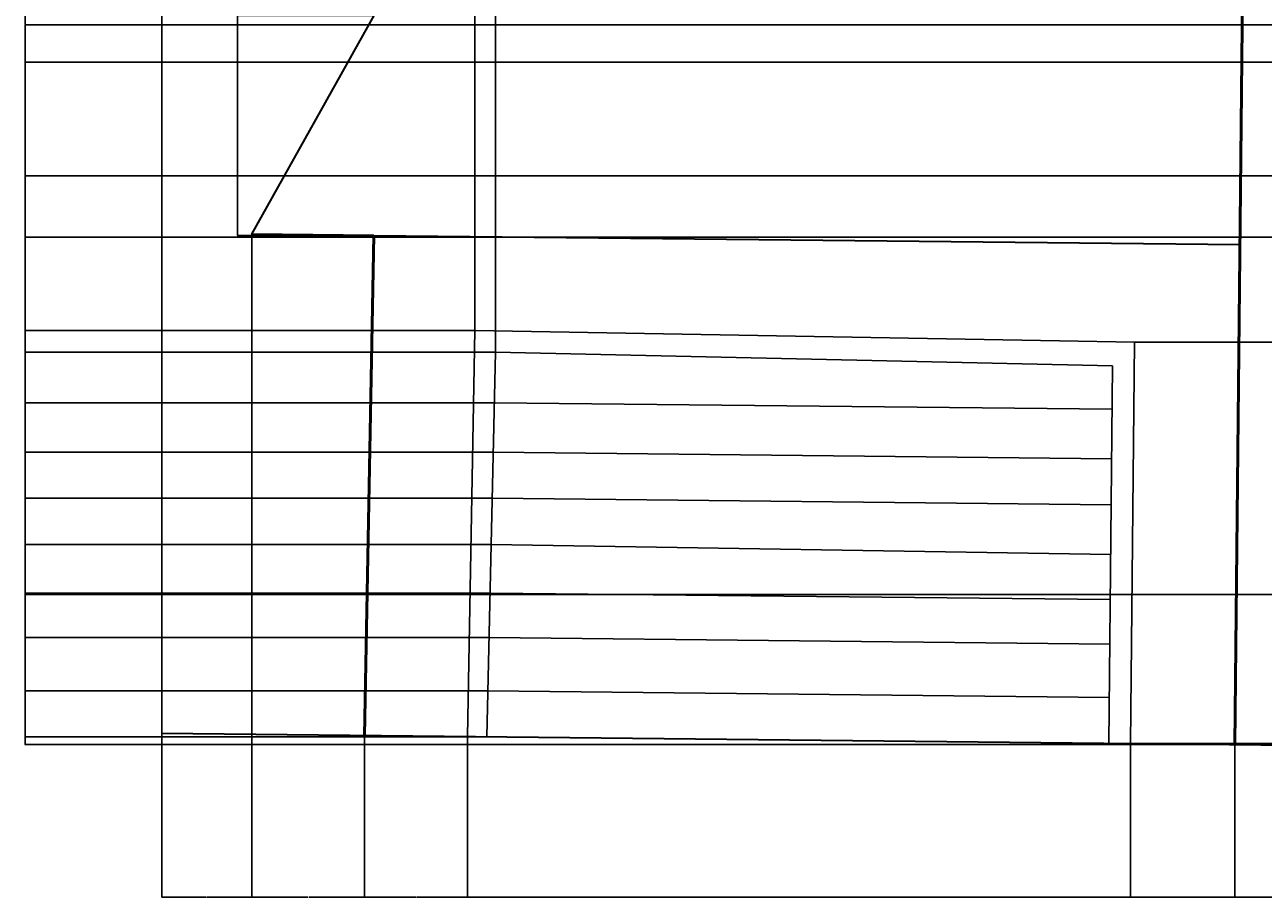
# Model space of a CAD drawing. Units: millimetres. Extents: x 1119 to 4262, y 854 to 2737.
# Tile 1 of 5: x 1119 to 2434, y 854 to 1780. Entities that reach past the tile are written whole.
import ezdxf

# ---------------------------------------------------------------- set-up
doc = ezdxf.new("R2010")
doc.units = ezdxf.units.MM
for name, color, linetype, lineweight in [('A-ANNO-DIMS', 2, 'Continuous', 18), ('A-DOOR', 3, 'Continuous', 25), ('A-ELEV', 8, 'Continuous', 35), ('A-ROOF', 1, 'Continuous', 35), ('A-WALL', 7, 'Continuous', 50)]:
    doc.layers.add(name, color=color, linetype=linetype, lineweight=lineweight)
doc.styles.get("Standard").update_dxf_attribs({"font": 'arial.ttf'})
doc.dimstyles.get("Standard").update_dxf_attribs({"dimtxt": 0.18, "dimasz": 0.18, "dimexe": 0.18, "dimexo": 0.0625, "dimgap": 0.09, "dimtad": 0, "dimtih": 1, "dimtoh": 1, "dimdec": 4, "dimzin": 0, "dimdsep": 46, "dimtxsty": 'Standard', "dimcen": 0.09, "dimadec": 0, "dimazin": 0, "dimtfac": 1, "dimtdec": 4, "dimtofl": 0, "dimtmove": 0, "dimatfit": 3, "dimfxl": 1, "dimtolj": 1, "dimtzin": 0, "dimarcsym": 0})

# ---------------------------------------------------------------- blocks, each defined once
blk = doc.blocks.new('*D1')
at = {"layer": 'A-ANNO-DIMS', "color": 0, "lineweight": -2, "transparency": 16777216}
for p, q in [((1360.1, 1558), (1360.1, 854.2)), ((1264.4, 1028.1), (1264.4, 854.2)), ((1264.5, 854.4), (1311.9, 854.4)), ((1360, 854.4), (1312.6, 854.4))]:
    blk.add_line(p, q, dxfattribs=at)
at = {"layer": 'A-ANNO-DIMS', "color": 0, "transparency": 16777216}
for points in [[(1264.5, 854.4), (1264.5, 854.3), (1264.4, 854.4)], [(1360, 854.4), (1360, 854.3), (1360.1, 854.4)]]:
    blk.add_solid(points, dxfattribs=at)
at = {"layer": 'Defpoints', "color": 0, "transparency": 16777216}
for p in [(1360.1, 1558.1), (1264.4, 1028.2), (1360.1, 854.4)]:
    blk.add_point(p, dxfattribs=at)
at = {"layer": 'A-ANNO-DIMS', "color": 0, "transparency": 16777216, "insert": (1312.2, 854.4), "char_height": 0.18, "attachment_point": 5}
blk.add_mtext('\\A1;95.78', dxfattribs=at)
blk = doc.blocks.new('*D2')
at = {"layer": 'A-ANNO-DIMS', "color": 0, "lineweight": -2, "transparency": 16777216}
for p, q in [((1360.1, 1558), (1360.1, 854.2)), ((1479.9, 1025.9), (1479.9, 854.2)), ((1360.3, 854.4), (1419.6, 854.4)), ((1479.7, 854.4), (1420.5, 854.4))]:
    blk.add_line(p, q, dxfattribs=at)
at = {"layer": 'A-ANNO-DIMS', "color": 0, "transparency": 16777216}
for points in [[(1360.3, 854.4), (1360.3, 854.3), (1360.1, 854.4)], [(1479.7, 854.4), (1479.7, 854.3), (1479.9, 854.4)]]:
    blk.add_solid(points, dxfattribs=at)
at = {"layer": 'Defpoints', "color": 0, "transparency": 16777216}
for p in [(1360.1, 1558.1), (1479.9, 1025.9), (1479.9, 854.4)]:
    blk.add_point(p, dxfattribs=at)
at = {"layer": 'A-ANNO-DIMS', "color": 0, "transparency": 16777216, "insert": (1420, 854.4), "char_height": 0.18, "attachment_point": 5}
blk.add_mtext('\\A1;119.76', dxfattribs=at)
blk = doc.blocks.new('*D3')
at = {"layer": 'A-ANNO-DIMS', "color": 0, "lineweight": -2, "transparency": 16777216}
for p, q in [((1479.9, 1025.9), (1479.9, 854.2)), ((1589.2, 1024.7), (1589.2, 854.2)), ((1480.1, 854.4), (1534.1, 854.4)), ((1589, 854.4), (1535, 854.4))]:
    blk.add_line(p, q, dxfattribs=at)
at = {"layer": 'A-ANNO-DIMS', "color": 0, "transparency": 16777216}
for points in [[(1480.1, 854.4), (1480.1, 854.3), (1479.9, 854.4)], [(1589, 854.4), (1589, 854.3), (1589.2, 854.4)]]:
    blk.add_solid(points, dxfattribs=at)
at = {"layer": 'Defpoints', "color": 0, "transparency": 16777216}
for p in [(1479.9, 1025.9), (1589.2, 1024.8), (1589.2, 854.4)]:
    blk.add_point(p, dxfattribs=at)
at = {"layer": 'A-ANNO-DIMS', "color": 0, "transparency": 16777216, "insert": (1534.6, 854.4), "char_height": 0.18, "attachment_point": 5}
blk.add_mtext('\\A1;109.32', dxfattribs=at)
blk = doc.blocks.new('*D4')
at = {"layer": 'A-ANNO-DIMS', "color": 0, "lineweight": -2, "transparency": 16777216}
for p, q in [((1589.2, 1024.7), (1589.2, 854.2)), ((2403.9, 1016.1), (2403.9, 854.2)), ((1589.4, 854.4), (1996.2, 854.4)), ((2403.7, 854.4), (1997, 854.4))]:
    blk.add_line(p, q, dxfattribs=at)
at = {"layer": 'A-ANNO-DIMS', "color": 0, "transparency": 16777216}
for points in [[(1589.4, 854.4), (1589.4, 854.3), (1589.2, 854.4)], [(2403.7, 854.4), (2403.7, 854.3), (2403.9, 854.4)]]:
    blk.add_solid(points, dxfattribs=at)
at = {"layer": 'Defpoints', "color": 0, "transparency": 16777216}
for p in [(1589.2, 1024.8), (2403.9, 1016.2), (2403.9, 854.4)]:
    blk.add_point(p, dxfattribs=at)
at = {"layer": 'A-ANNO-DIMS', "color": 0, "transparency": 16777216, "insert": (1996.6, 854.4), "char_height": 0.18, "attachment_point": 5}
blk.add_mtext('\\A1;814.7', dxfattribs=at)
blk = doc.blocks.new('*D5')
at = {"layer": 'A-ANNO-DIMS', "color": 0, "lineweight": -2, "transparency": 16777216}
for p, q in [((2537.2, 1175.4), (2537.2, 854.2)), ((2403.9, 1016.1), (2403.9, 854.2)), ((2404.1, 854.4), (2470.2, 854.4)), ((2537, 854.4), (2470.9, 854.4))]:
    blk.add_line(p, q, dxfattribs=at)
at = {"layer": 'A-ANNO-DIMS', "color": 0, "transparency": 16777216}
for points in [[(2404.1, 854.4), (2404.1, 854.3), (2403.9, 854.4)], [(2537, 854.4), (2537, 854.3), (2537.2, 854.4)]]:
    blk.add_solid(points, dxfattribs=at)
at = {"layer": 'Defpoints', "color": 0, "transparency": 16777216}
for p in [(2537.2, 1175.4), (2403.9, 1016.2), (2537.2, 854.4)]:
    blk.add_point(p, dxfattribs=at)
at = {"layer": 'A-ANNO-DIMS', "color": 0, "transparency": 16777216, "insert": (2470.5, 854.4), "char_height": 0.18, "attachment_point": 5}
blk.add_mtext('\\A1;133.3', dxfattribs=at)
blk = doc.blocks.new('*D13')
at = {"layer": 'A-ANNO-DIMS', "color": 0, "lineweight": -2, "transparency": 16777216}
for p, q in [((1264.4, 1028.3), (1264.4, 2737.1)), ((1264.5, 2737), (2690.1, 2737)), ((4116.6, 2737), (2691, 2737)), ((4116.8, 2249.8), (4116.8, 2737.1))]:
    blk.add_line(p, q, dxfattribs=at)
at = {"layer": 'A-ANNO-DIMS', "color": 0, "transparency": 16777216}
for points in [[(1264.5, 2737), (1264.5, 2736.9), (1264.4, 2737)], [(4116.6, 2737), (4116.6, 2736.9), (4116.8, 2737)]]:
    blk.add_solid(points, dxfattribs=at)
at = {"layer": 'Defpoints', "color": 0, "transparency": 16777216}
for p in [(4116.8, 2737), (4116.8, 2249.7), (1264.4, 1028.2)]:
    blk.add_point(p, dxfattribs=at)
at = {"layer": 'A-ANNO-DIMS', "color": 0, "transparency": 16777216, "insert": (2690.6, 2737), "char_height": 0.18, "attachment_point": 5}
blk.add_mtext('\\A1;2852.4', dxfattribs=at)
blk = doc.blocks.new('*D31')
at = {"layer": 'A-ANNO-DIMS', "color": 0, "lineweight": -2, "transparency": 16777216}
for p, q in [((2537.1, 1175.4), (1119.2, 1175.4)), ((1119.4, 1175.3), (1119.4, 1096)), ((1119.4, 1016.4), (1119.4, 1095.6)), ((2403.8, 1016.2), (1119.2, 1016.2))]:
    blk.add_line(p, q, dxfattribs=at)
at = {"layer": 'A-ANNO-DIMS', "color": 0, "transparency": 16777216}
for points in [[(1119.3, 1175.3), (1119.4, 1175.3), (1119.4, 1175.4)], [(1119.3, 1016.4), (1119.4, 1016.4), (1119.4, 1016.2)]]:
    blk.add_solid(points, dxfattribs=at)
at = {"layer": 'Defpoints', "color": 0, "transparency": 16777216}
for p in [(1119.4, 1175.4), (2537.2, 1175.4), (2403.9, 1016.2)]:
    blk.add_point(p, dxfattribs=at)
at = {"layer": 'A-ANNO-DIMS', "color": 0, "transparency": 16777216, "insert": (1119.4, 1095.8), "char_height": 0.18, "attachment_point": 5}
blk.add_mtext('\\A1;159.26', dxfattribs=at)
blk = doc.blocks.new('*D32')
at = {"layer": 'A-ANNO-DIMS', "color": 0, "lineweight": -2, "transparency": 16777216}
for p, q in [((2537.1, 1554.7), (1119.2, 1554.7)), ((1119.4, 1554.5), (1119.4, 1365.2)), ((1119.4, 1175.6), (1119.4, 1364.9)), ((2537.1, 1175.4), (1119.2, 1175.4))]:
    blk.add_line(p, q, dxfattribs=at)
at = {"layer": 'A-ANNO-DIMS', "color": 0, "transparency": 16777216}
for points in [[(1119.3, 1554.5), (1119.4, 1554.5), (1119.4, 1554.7)], [(1119.3, 1175.6), (1119.4, 1175.6), (1119.4, 1175.4)]]:
    blk.add_solid(points, dxfattribs=at)
at = {"layer": 'Defpoints', "color": 0, "transparency": 16777216}
for p in [(1119.4, 1554.7), (2537.2, 1554.7), (2537.2, 1175.4)]:
    blk.add_point(p, dxfattribs=at)
at = {"layer": 'A-ANNO-DIMS', "color": 0, "transparency": 16777216, "insert": (1119.4, 1365.1), "char_height": 0.18, "attachment_point": 5}
blk.add_mtext('\\A1;379.2', dxfattribs=at)
blk = doc.blocks.new('*D33')
at = {"layer": 'A-ANNO-DIMS', "color": 0, "lineweight": -2, "transparency": 16777216}
for p, q in [((2537.1, 1780.3), (1119.2, 1780.3)), ((1119.4, 1780.1), (1119.4, 1667.7)), ((1119.4, 1554.9), (1119.4, 1667.3)), ((2537.1, 1554.7), (1119.2, 1554.7))]:
    blk.add_line(p, q, dxfattribs=at)
at = {"layer": 'A-ANNO-DIMS', "color": 0, "transparency": 16777216}
for points in [[(1119.3, 1780.1), (1119.4, 1780.1), (1119.4, 1780.3)], [(1119.3, 1554.9), (1119.4, 1554.9), (1119.4, 1554.7)]]:
    blk.add_solid(points, dxfattribs=at)
at = {"layer": 'Defpoints', "color": 0, "transparency": 16777216}
for p in [(1119.4, 1780.3), (2537.2, 1780.3), (2537.2, 1554.7)]:
    blk.add_point(p, dxfattribs=at)
at = {"layer": 'A-ANNO-DIMS', "color": 0, "transparency": 16777216, "insert": (1119.4, 1667.5), "char_height": 0.18, "attachment_point": 5}
blk.add_mtext('\\A1;225.6', dxfattribs=at)
blk = doc.blocks.new('*D34')
at = {"layer": 'A-ANNO-DIMS', "color": 0, "lineweight": -2, "transparency": 16777216}
for p, q in [((2537.1, 2135.5), (1119.2, 2135.5)), ((1119.4, 2135.3), (1119.4, 1958.1)), ((1119.4, 1780.5), (1119.4, 1957.7)), ((2537.1, 1780.3), (1119.2, 1780.3))]:
    blk.add_line(p, q, dxfattribs=at)
at = {"layer": 'A-ANNO-DIMS', "color": 0, "transparency": 16777216}
for points in [[(1119.3, 2135.3), (1119.4, 2135.3), (1119.4, 2135.5)], [(1119.3, 1780.5), (1119.4, 1780.5), (1119.4, 1780.3)]]:
    blk.add_solid(points, dxfattribs=at)
at = {"layer": 'Defpoints', "color": 0, "transparency": 16777216}
for p in [(1119.4, 2135.5), (2537.2, 2135.5), (2537.2, 1780.3)]:
    blk.add_point(p, dxfattribs=at)
at = {"layer": 'A-ANNO-DIMS', "color": 0, "transparency": 16777216, "insert": (1119.4, 1957.9), "char_height": 0.18, "attachment_point": 5}
blk.add_mtext('\\A1;355.2', dxfattribs=at)
blk = doc.blocks.new('*D46')
at = {"layer": 'A-ANNO-DIMS', "color": 0, "lineweight": -2, "transparency": 16777216}
for p, q in [((1489.8, 1790.1), (1344.7, 1790.2)), ((1344.9, 1790), (1344.8, 1673.7)), ((1344.8, 1556.9), (1344.8, 1673.3)), ((1489.7, 1556.7), (1344.6, 1556.8))]:
    blk.add_line(p, q, dxfattribs=at)
at = {"layer": 'A-ANNO-DIMS', "color": 0, "transparency": 16777216}
for points in [[(1344.8, 1790), (1344.9, 1790), (1344.9, 1790.2)], [(1344.7, 1556.9), (1344.8, 1556.9), (1344.8, 1556.8)]]:
    blk.add_solid(points, dxfattribs=at)
at = {"layer": 'Defpoints', "color": 0, "transparency": 16777216}
for p in [(1344.9, 1790.2), (1489.9, 1790.1), (1489.8, 1556.7)]:
    blk.add_point(p, dxfattribs=at)
at = {"layer": 'A-ANNO-DIMS', "color": 0, "transparency": 16777216, "insert": (1344.8, 1673.5), "char_height": 0.18, "attachment_point": 5}
blk.add_mtext('\\A1;233.4', dxfattribs=at)
blk = doc.blocks.new('*D67')
at = {"layer": 'A-ANNO-DIMS', "color": 0, "lineweight": -2, "transparency": 16777216}
for p, q in [((3217.2, 1740.6), (1119.2, 1740.6)), ((1119.4, 1740.4), (1119.4, 1680.5)), ((1119.4, 1620.3), (1119.4, 1680.1)), ((3126.2, 1620.1), (1119.2, 1620.1))]:
    blk.add_line(p, q, dxfattribs=at)
at = {"layer": 'A-ANNO-DIMS', "color": 0, "transparency": 16777216}
for points in [[(1119.3, 1740.4), (1119.4, 1740.4), (1119.4, 1740.6)], [(1119.3, 1620.3), (1119.4, 1620.3), (1119.4, 1620.1)]]:
    blk.add_solid(points, dxfattribs=at)
at = {"layer": 'Defpoints', "color": 0, "transparency": 16777216}
for p in [(1119.4, 1740.6), (3217.3, 1740.6), (3126.3, 1620.1)]:
    blk.add_point(p, dxfattribs=at)
at = {"layer": 'A-ANNO-DIMS', "color": 0, "transparency": 16777216, "insert": (1119.4, 1680.3), "char_height": 0.18, "attachment_point": 5}
blk.add_mtext('\\A1;120.48', dxfattribs=at)
blk = doc.blocks.new('*D68')
at = {"layer": 'A-ANNO-DIMS', "color": 0, "lineweight": -2, "transparency": 16777216}
for p, q in [((1589.2, 1024.7), (1589.2, 854.2)), ((2293.1, 1017.3), (2293.1, 854.2)), ((1589.4, 854.4), (1940.8, 854.4)), ((2292.9, 854.4), (1941.5, 854.4))]:
    blk.add_line(p, q, dxfattribs=at)
at = {"layer": 'A-ANNO-DIMS', "color": 0, "transparency": 16777216}
for points in [[(1589.4, 854.4), (1589.4, 854.3), (1589.2, 854.4)], [(2292.9, 854.4), (2292.9, 854.3), (2293.1, 854.4)]]:
    blk.add_solid(points, dxfattribs=at)
at = {"layer": 'Defpoints', "color": 0, "transparency": 16777216}
for p in [(1589.2, 1024.8), (2293.1, 1017.4), (2293.1, 854.4)]:
    blk.add_point(p, dxfattribs=at)
at = {"layer": 'A-ANNO-DIMS', "color": 0, "transparency": 16777216, "insert": (1941.1, 854.4), "char_height": 0.18, "attachment_point": 5}
blk.add_mtext('\\A1;703.8', dxfattribs=at)
blk = doc.blocks.new('*D69')
at = {"layer": 'A-ANNO-DIMS', "color": 0, "lineweight": -2, "transparency": 16777216}
for p, q in [((1610.8, 1073.3), (1119.2, 1073.3)), ((1119.4, 1073.1), (1119.4, 1049.1)), ((1119.4, 1024.7), (1119.4, 1048.7)), ((1609.7, 1024.6), (1119.2, 1024.6))]:
    blk.add_line(p, q, dxfattribs=at)
at = {"layer": 'A-ANNO-DIMS', "color": 0, "transparency": 16777216}
for points in [[(1119.3, 1073.1), (1119.4, 1073.1), (1119.4, 1073.3)], [(1119.3, 1024.7), (1119.4, 1024.7), (1119.4, 1024.6)]]:
    blk.add_solid(points, dxfattribs=at)
at = {"layer": 'Defpoints', "color": 0, "transparency": 16777216}
for p in [(1119.4, 1073.3), (1610.8, 1073.3), (1609.7, 1024.6)]:
    blk.add_point(p, dxfattribs=at)
at = {"layer": 'A-ANNO-DIMS', "color": 0, "transparency": 16777216, "insert": (1119.4, 1048.9), "char_height": 0.18, "attachment_point": 5}
blk.add_mtext('\\A1;48.71', dxfattribs=at)
blk = doc.blocks.new('*D70')
at = {"layer": 'A-ANNO-DIMS', "color": 0, "lineweight": -2, "transparency": 16777216}
for p, q in [((1612, 1129.9), (1119.2, 1129.9)), ((1119.4, 1129.7), (1119.4, 1101.8)), ((1119.4, 1073.5), (1119.4, 1101.4)), ((1610.8, 1073.3), (1119.2, 1073.3))]:
    blk.add_line(p, q, dxfattribs=at)
at = {"layer": 'A-ANNO-DIMS', "color": 0, "transparency": 16777216}
for points in [[(1119.3, 1129.7), (1119.4, 1129.7), (1119.4, 1129.9)], [(1119.3, 1073.5), (1119.4, 1073.5), (1119.4, 1073.3)]]:
    blk.add_solid(points, dxfattribs=at)
at = {"layer": 'Defpoints', "color": 0, "transparency": 16777216}
for p in [(1119.4, 1129.9), (1612.1, 1129.9), (1610.8, 1073.3)]:
    blk.add_point(p, dxfattribs=at)
at = {"layer": 'A-ANNO-DIMS', "color": 0, "transparency": 16777216, "insert": (1119.4, 1101.6), "char_height": 0.18, "attachment_point": 5}
blk.add_mtext('\\A1;56.61', dxfattribs=at)
blk = doc.blocks.new('*D71')
at = {"layer": 'A-ANNO-DIMS', "color": 0, "lineweight": -2, "transparency": 16777216}
for p, q in [((1613, 1177.1), (1119.2, 1177.1)), ((1119.4, 1176.9), (1119.4, 1153.7)), ((1119.4, 1130.1), (1119.4, 1153.3)), ((1612, 1129.9), (1119.2, 1129.9))]:
    blk.add_line(p, q, dxfattribs=at)
at = {"layer": 'A-ANNO-DIMS', "color": 0, "transparency": 16777216}
for points in [[(1119.3, 1176.9), (1119.4, 1176.9), (1119.4, 1177.1)], [(1119.3, 1130.1), (1119.4, 1130.1), (1119.4, 1129.9)]]:
    blk.add_solid(points, dxfattribs=at)
at = {"layer": 'Defpoints', "color": 0, "transparency": 16777216}
for p in [(1119.4, 1177.1), (1613.1, 1177.1), (1612.1, 1129.9)]:
    blk.add_point(p, dxfattribs=at)
at = {"layer": 'A-ANNO-DIMS', "color": 0, "transparency": 16777216, "insert": (1119.4, 1153.5), "char_height": 0.18, "attachment_point": 5}
blk.add_mtext('\\A1;47.21', dxfattribs=at)
blk = doc.blocks.new('*D72')
at = {"layer": 'A-ANNO-DIMS', "color": 0, "lineweight": -2, "transparency": 16777216}
for p, q in [((1614.2, 1228.7), (1119.2, 1228.7)), ((1119.4, 1228.5), (1119.4, 1203.1)), ((1119.4, 1177.3), (1119.4, 1202.7)), ((1613, 1177.1), (1119.2, 1177.1))]:
    blk.add_line(p, q, dxfattribs=at)
at = {"layer": 'A-ANNO-DIMS', "color": 0, "transparency": 16777216}
for points in [[(1119.3, 1228.5), (1119.4, 1228.5), (1119.4, 1228.7)], [(1119.3, 1177.3), (1119.4, 1177.3), (1119.4, 1177.1)]]:
    blk.add_solid(points, dxfattribs=at)
at = {"layer": 'Defpoints', "color": 0, "transparency": 16777216}
for p in [(1119.4, 1228.7), (1614.2, 1228.7), (1613.1, 1177.1)]:
    blk.add_point(p, dxfattribs=at)
at = {"layer": 'A-ANNO-DIMS', "color": 0, "transparency": 16777216, "insert": (1119.4, 1202.9), "char_height": 0.18, "attachment_point": 5}
blk.add_mtext('\\A1;51.62', dxfattribs=at)
blk = doc.blocks.new('*D73')
at = {"layer": 'A-ANNO-DIMS', "color": 0, "lineweight": -2, "transparency": 16777216}
for p, q in [((1615.3, 1277.7), (1119.2, 1277.7)), ((1119.4, 1277.5), (1119.4, 1253.4)), ((1119.4, 1228.9), (1119.4, 1253)), ((1614.2, 1228.7), (1119.2, 1228.7))]:
    blk.add_line(p, q, dxfattribs=at)
at = {"layer": 'A-ANNO-DIMS', "color": 0, "transparency": 16777216}
for points in [[(1119.3, 1277.5), (1119.4, 1277.5), (1119.4, 1277.7)], [(1119.3, 1228.9), (1119.4, 1228.9), (1119.4, 1228.7)]]:
    blk.add_solid(points, dxfattribs=at)
at = {"layer": 'Defpoints', "color": 0, "transparency": 16777216}
for p in [(1119.4, 1277.7), (1615.3, 1277.7), (1614.2, 1228.7)]:
    blk.add_point(p, dxfattribs=at)
at = {"layer": 'A-ANNO-DIMS', "color": 0, "transparency": 16777216, "insert": (1119.4, 1253.2), "char_height": 0.18, "attachment_point": 5}
blk.add_mtext('\\A1;48.98', dxfattribs=at)
blk = doc.blocks.new('*D74')
at = {"layer": 'A-ANNO-DIMS', "color": 0, "lineweight": -2, "transparency": 16777216}
for p, q in [((1616.3, 1326.5), (1119.2, 1326.5)), ((1119.4, 1326.3), (1119.4, 1302.3)), ((1119.4, 1277.9), (1119.4, 1301.9)), ((1615.3, 1277.7), (1119.2, 1277.7))]:
    blk.add_line(p, q, dxfattribs=at)
at = {"layer": 'A-ANNO-DIMS', "color": 0, "transparency": 16777216}
for points in [[(1119.3, 1326.3), (1119.4, 1326.3), (1119.4, 1326.5)], [(1119.3, 1277.9), (1119.4, 1277.9), (1119.4, 1277.7)]]:
    blk.add_solid(points, dxfattribs=at)
at = {"layer": 'Defpoints', "color": 0, "transparency": 16777216}
for p in [(1119.4, 1326.5), (1616.4, 1326.5), (1615.3, 1277.7)]:
    blk.add_point(p, dxfattribs=at)
at = {"layer": 'A-ANNO-DIMS', "color": 0, "transparency": 16777216, "insert": (1119.4, 1302.1), "char_height": 0.18, "attachment_point": 5}
blk.add_mtext('\\A1;48.82', dxfattribs=at)
blk = doc.blocks.new('*D75')
at = {"layer": 'A-ANNO-DIMS', "color": 0, "lineweight": -2, "transparency": 16777216}
for p, q in [((1617.5, 1379.1), (1119.2, 1379.1)), ((1119.4, 1378.9), (1119.4, 1353)), ((1119.4, 1326.7), (1119.4, 1352.6)), ((1616.3, 1326.5), (1119.2, 1326.5))]:
    blk.add_line(p, q, dxfattribs=at)
at = {"layer": 'A-ANNO-DIMS', "color": 0, "transparency": 16777216}
for points in [[(1119.3, 1378.9), (1119.4, 1378.9), (1119.4, 1379.1)], [(1119.3, 1326.7), (1119.4, 1326.7), (1119.4, 1326.5)]]:
    blk.add_solid(points, dxfattribs=at)
at = {"layer": 'Defpoints', "color": 0, "transparency": 16777216}
for p in [(1119.4, 1379.1), (1617.6, 1379.1), (1616.4, 1326.5)]:
    blk.add_point(p, dxfattribs=at)
at = {"layer": 'A-ANNO-DIMS', "color": 0, "transparency": 16777216, "insert": (1119.4, 1352.8), "char_height": 0.18, "attachment_point": 5}
blk.add_mtext('\\A1;52.61', dxfattribs=at)
blk = doc.blocks.new('*D76')
at = {"layer": 'A-ANNO-DIMS', "color": 0, "lineweight": -2, "transparency": 16777216}
for p, q in [((1618.7, 1432.9), (1119.2, 1432.9)), ((1119.4, 1432.7), (1119.4, 1406.2)), ((1119.4, 1379.3), (1119.4, 1405.8)), ((1617.5, 1379.1), (1119.2, 1379.1))]:
    blk.add_line(p, q, dxfattribs=at)
at = {"layer": 'A-ANNO-DIMS', "color": 0, "transparency": 16777216}
for points in [[(1119.3, 1432.7), (1119.4, 1432.7), (1119.4, 1432.9)], [(1119.3, 1379.3), (1119.4, 1379.3), (1119.4, 1379.1)]]:
    blk.add_solid(points, dxfattribs=at)
at = {"layer": 'Defpoints', "color": 0, "transparency": 16777216}
for p in [(1119.4, 1432.9), (1618.7, 1432.9), (1617.6, 1379.1)]:
    blk.add_point(p, dxfattribs=at)
at = {"layer": 'A-ANNO-DIMS', "color": 0, "transparency": 16777216, "insert": (1119.4, 1406), "char_height": 0.18, "attachment_point": 5}
blk.add_mtext('\\A1;53.75', dxfattribs=at)
blk = doc.blocks.new('*D77')
at = {"layer": 'A-ANNO-DIMS', "color": 0, "lineweight": -2, "transparency": 16777216}
for p, q in [((1596.9, 1455.9), (1119.2, 1455.9)), ((1119.4, 1455.8), (1119.4, 1444.6)), ((1119.4, 1433), (1119.4, 1444.2)), ((1618.7, 1432.9), (1119.2, 1432.9))]:
    blk.add_line(p, q, dxfattribs=at)
at = {"layer": 'A-ANNO-DIMS', "color": 0, "transparency": 16777216}
for points in [[(1119.3, 1455.8), (1119.4, 1455.8), (1119.4, 1455.9)], [(1119.3, 1433), (1119.4, 1433), (1119.4, 1432.9)]]:
    blk.add_solid(points, dxfattribs=at)
at = {"layer": 'Defpoints', "color": 0, "transparency": 16777216}
for p in [(1119.4, 1455.9), (1596.9, 1455.9), (1618.7, 1432.9)]:
    blk.add_point(p, dxfattribs=at)
at = {"layer": 'A-ANNO-DIMS', "color": 0, "transparency": 16777216, "insert": (1119.4, 1444.4), "char_height": 0.18, "attachment_point": 5}
blk.add_mtext('\\A1;23.082', dxfattribs=at)
blk = doc.blocks.new('*D78')
at = {"layer": 'A-ANNO-DIMS', "color": 0, "lineweight": -2, "transparency": 16777216}
for p, q in [((2297.6, 1443.4), (4262, 1443.4)), ((4261.8, 1443.2), (4261.8, 1230.6)), ((4261.8, 1017.5), (4261.8, 1230.2)), ((2293.1, 1017.4), (4262, 1017.4))]:
    blk.add_line(p, q, dxfattribs=at)
at = {"layer": 'A-ANNO-DIMS', "color": 0, "transparency": 16777216}
for points in [[(4261.8, 1443.2), (4261.8, 1443.2), (4261.8, 1443.4)], [(4261.8, 1017.5), (4261.8, 1017.5), (4261.8, 1017.4)]]:
    blk.add_solid(points, dxfattribs=at)
at = {"layer": 'Defpoints', "color": 0, "transparency": 16777216}
for p in [(2297.6, 1443.4), (4261.8, 1443.4), (2293.1, 1017.4)]:
    blk.add_point(p, dxfattribs=at)
at = {"layer": 'A-ANNO-DIMS', "color": 0, "transparency": 16777216, "insert": (4261.8, 1230.4), "char_height": 0.18, "attachment_point": 5}
blk.add_mtext('\\A1;426.06', dxfattribs=at)
blk = doc.blocks.new('*D79')
at = {"layer": 'A-ANNO-DIMS', "color": 0, "lineweight": -2, "transparency": 16777216}
for p, q in [((1596.9, 1456), (1596.9, 2737.1)), ((1597.1, 2737), (1607.4, 2737)), ((1618.6, 2737), (1608.3, 2737)), ((1618.7, 1432.9), (1618.7, 2737.1))]:
    blk.add_line(p, q, dxfattribs=at)
at = {"layer": 'A-ANNO-DIMS', "color": 0, "transparency": 16777216}
for points in [[(1597.1, 2737), (1597.1, 2736.9), (1596.9, 2737)], [(1618.6, 2737), (1618.6, 2736.9), (1618.7, 2737)]]:
    blk.add_solid(points, dxfattribs=at)
at = {"layer": 'Defpoints', "color": 0, "transparency": 16777216}
for p in [(1618.7, 2737), (1596.9, 1455.9), (1618.7, 1432.9)]:
    blk.add_point(p, dxfattribs=at)
at = {"layer": 'A-ANNO-DIMS', "color": 0, "transparency": 16777216, "insert": (1607.8, 2737), "char_height": 0.18, "attachment_point": 5}
blk.add_mtext('\\A1;21.813', dxfattribs=at)

msp = doc.modelspace()

# ---------------------------------------------------------------- linework, layer by layer
at = {"layer": 'A-DOOR'}
for p, q in [((1589.2208, 1024.7774), (1596.9363, 1455.9499)), ((1596.9363, 1455.9499), (2217.8713, 1444.8386)), ((2217.8713, 1444.8386), (2297.5614, 1443.4126)), ((2297.5614, 1443.4126), (2293.0699, 1017.3574)), ((1609.7488, 1024.561), (1618.7498, 1432.8675)), ((1618.7498, 1432.8675), (2274.2595, 1418.4171)), ((2274.2595, 1418.4171), (2270.034, 1017.6003)), ((1617.5649, 1379.1198), (2273.7723, 1372.202)), ((1616.4052, 1326.5123), (2273.2176, 1319.5882)), ((1615.329, 1277.6935), (2272.7029, 1270.7635)), ((1614.2493, 1228.7143), (2272.1468, 1218.0087)), ((1613.1114, 1177.0964), (2271.6423, 1170.1541)), ((1612.0707, 1129.8866), (2271.1445, 1122.9387)), ((1610.8227, 1073.2758), (2270.5477, 1066.321))]:
    msp.add_line(p, q, dxfattribs=at)
at = {"layer": 'A-ELEV'}
msp.add_line((1264.3595, 1028.2021), (4000.5454, 999.3572), dxfattribs=at)
at = {"layer": 'A-ROOF'}
for p, q in [((1360.1359, 1558.0571), (1489.8677, 1790.1098)), ((1489.7567, 1556.6906), (1360.1359, 1558.0571)), ((1489.7567, 1556.6906), (2409.4887, 1546.9948))]:
    msp.add_line(p, q, dxfattribs=at)
at = {"layer": 'A-WALL'}
for p, q in [((2416.9805, 2257.6545), (2403.8929, 1016.1891)), ((1479.8981, 1025.9299), (1489.7567, 1556.6906))]:
    msp.add_line(p, q, dxfattribs=at)

# ---------------------------------------------------------------- dimensions: what is measured, and where the dimension line sits
at = {"layer": 'A-ANNO-DIMS'}
for base, p1, p2, override, picture, middle in [((4116.7957, 2736.9672), (1264.3595, 1028.2021), (4116.7957, 2249.7378), {"dimdec": 1, "dimlfac": 1, "dimrnd": 0, "dimzin": 0, "dimdsep": 46, "dimlunit": 2}, '*D13', (2690.5776, 2736.9672)), ((1618.74978, 2736.96722), (1596.93635, 1455.94989), (1618.74978, 1432.86755), {"dimdec": 3, "dimlfac": 1, "dimrnd": 0, "dimzin": 0, "dimdsep": 46, "dimlunit": 2}, '*D79', (1607.84307, 2736.96722)), ((1360.1359, 854.3572), (1264.3595, 1028.2021), (1360.1359, 1558.0571), {"dimdec": 2, "dimlfac": 1, "dimrnd": 0, "dimzin": 0, "dimdsep": 46, "dimlunit": 2}, '*D1', (1312.2477, 854.3572)), ((1479.8981, 854.3572), (1360.1359, 1558.0571), (1479.8981, 1025.9299), {"dimdec": 2, "dimlfac": 1, "dimrnd": 0, "dimzin": 0, "dimdsep": 46, "dimlunit": 2}, '*D2', (1420.017, 854.3572)), ((2537.1892, 854.3572), (2403.8929, 1016.1891), (2537.1892, 1175.4491), {"dimdec": 1, "dimlfac": 1, "dimrnd": 0, "dimzin": 0, "dimdsep": 46, "dimlunit": 2}, '*D5', (2470.5411, 854.3572)), ((1589.2208, 854.3572), (1479.8981, 1025.9299), (1589.2208, 1024.7774), {"dimdec": 2, "dimlfac": 1, "dimrnd": 0, "dimzin": 0, "dimdsep": 46, "dimlunit": 2}, '*D3', (1534.5594, 854.3572)), ((2403.8929, 854.3572), (1589.2208, 1024.7774), (2403.8929, 1016.1891), {"dimdec": 1, "dimlfac": 1, "dimrnd": 0, "dimzin": 0, "dimdsep": 46, "dimlunit": 2}, '*D4', (1996.5568, 854.3572)), ((2293.0699, 854.3572), (1589.2208, 1024.7774), (2293.0699, 1017.3574), {"dimdec": 1, "dimlfac": 1, "dimrnd": 0, "dimzin": 0, "dimdsep": 46, "dimlunit": 2}, '*D68', (1941.1453, 854.3572))]:
    dim = msp.add_linear_dim(base=base, p1=p1, p2=p2, dimstyle='Standard', override=override, dxfattribs=at)
    dim.commit()
    dim.dimension.update_dxf_attribs({"geometry": picture, "text_midpoint": middle})
for base, p1, p2, angle, override, picture, middle in [((1119.3595, 2135.5085), (2537.1892, 1780.2865), (2537.1892, 2135.5085), 90, {"dimdec": 1, "dimlfac": 1, "dimrnd": 0, "dimzin": 0, "dimdsep": 46, "dimlunit": 2}, '*D34', (1119.3595, 1957.8975)), ((1344.8677, 1790.1787), (1489.7567, 1556.6906), (1489.8677, 1790.1098), 89.9727569, {"dimdec": 1, "dimlfac": 1, "dimrnd": 0, "dimzin": 0, "dimdsep": 46, "dimlunit": 2}, '*D46', (1344.8122, 1673.4691)), ((1119.3595, 1780.2865), (2537.1892, 1554.6726), (2537.1892, 1780.2865), 90, {"dimdec": 1, "dimlfac": 1, "dimrnd": 0, "dimzin": 0, "dimdsep": 46, "dimlunit": 2}, '*D33', (1119.3595, 1667.4795)), ((1119.3595, 1740.5658), (3126.2541, 1620.0857), (3217.2823, 1740.5658), 90, {"dimdec": 2, "dimlfac": 1, "dimrnd": 0, "dimzin": 0, "dimdsep": 46, "dimlunit": 2}, '*D67', (1119.3595, 1680.3258)), ((1119.3595, 1554.6726), (2537.1892, 1175.4491), (2537.1892, 1554.6726), 90, {"dimdec": 1, "dimlfac": 1, "dimrnd": 0, "dimzin": 0, "dimdsep": 46, "dimlunit": 2}, '*D32', (1119.3595, 1365.0608)), ((1119.3595, 1455.9499), (1618.7498, 1432.8675), (1596.9363, 1455.9499), 90, {"dimdec": 3, "dimlfac": 1, "dimrnd": 0, "dimzin": 0, "dimdsep": 46, "dimlunit": 2}, '*D77', (1119.3595, 1444.4087)), ((4261.7957, 1443.4126), (2293.0699, 1017.3574), (2297.5614, 1443.4126), 90, {"dimdec": 2, "dimlfac": 1, "dimrnd": 0, "dimzin": 0, "dimdsep": 46, "dimlunit": 2}, '*D78', (4261.7957, 1230.385)), ((1119.3595, 1432.8675), (1617.5649, 1379.1198), (1618.7498, 1432.8675), 90, {"dimdec": 2, "dimlfac": 1, "dimrnd": 0, "dimzin": 0, "dimdsep": 46, "dimlunit": 2}, '*D76', (1119.3595, 1405.9937)), ((1119.3595, 1379.1198), (1616.4052, 1326.5123), (1617.5649, 1379.1198), 90, {"dimdec": 2, "dimlfac": 1, "dimrnd": 0, "dimzin": 0, "dimdsep": 46, "dimlunit": 2}, '*D75', (1119.3595, 1352.816)), ((1119.3595, 1326.5123), (1615.329, 1277.6935), (1616.4052, 1326.5123), 90, {"dimdec": 2, "dimlfac": 1, "dimrnd": 0, "dimzin": 0, "dimdsep": 46, "dimlunit": 2}, '*D74', (1119.3595, 1302.1029)), ((1119.3595, 1277.6935), (1614.2493, 1228.7143), (1615.329, 1277.6935), 90, {"dimdec": 2, "dimlfac": 1, "dimrnd": 0, "dimzin": 0, "dimdsep": 46, "dimlunit": 2}, '*D73', (1119.3595, 1253.2039)), ((1119.3595, 1228.7143), (1613.1114, 1177.0964), (1614.2493, 1228.7143), 90, {"dimdec": 2, "dimlfac": 1, "dimrnd": 0, "dimzin": 0, "dimdsep": 46, "dimlunit": 2}, '*D72', (1119.3595, 1202.9053)), ((1119.3595, 1175.4491), (2403.8929, 1016.1891), (2537.1892, 1175.4491), 90, {"dimdec": 2, "dimlfac": 1, "dimrnd": 0, "dimzin": 0, "dimdsep": 46, "dimlunit": 2}, '*D31', (1119.3595, 1095.8191)), ((1119.3595, 1177.0964), (1612.0707, 1129.8866), (1613.1114, 1177.0964), 90, {"dimdec": 2, "dimlfac": 1, "dimrnd": 0, "dimzin": 0, "dimdsep": 46, "dimlunit": 2}, '*D71', (1119.3595, 1153.4915)), ((1119.3595, 1129.8866), (1610.8227, 1073.2758), (1612.0707, 1129.8866), 90, {"dimdec": 2, "dimlfac": 1, "dimrnd": 0, "dimzin": 0, "dimdsep": 46, "dimlunit": 2}, '*D70', (1119.3595, 1101.5812)), ((1119.3595, 1073.2758), (1609.7488, 1024.561), (1610.8227, 1073.2758), 90, {"dimdec": 2, "dimlfac": 1, "dimrnd": 0, "dimzin": 0, "dimdsep": 46, "dimlunit": 2}, '*D69', (1119.3595, 1048.9184))]:
    dim = msp.add_linear_dim(base=base, p1=p1, p2=p2, angle=angle, dimstyle='Standard', override=override, dxfattribs=at)
    dim.commit()
    dim.dimension.update_dxf_attribs({"geometry": picture, "text_midpoint": middle})

doc.saveas('drawing.dxf')
